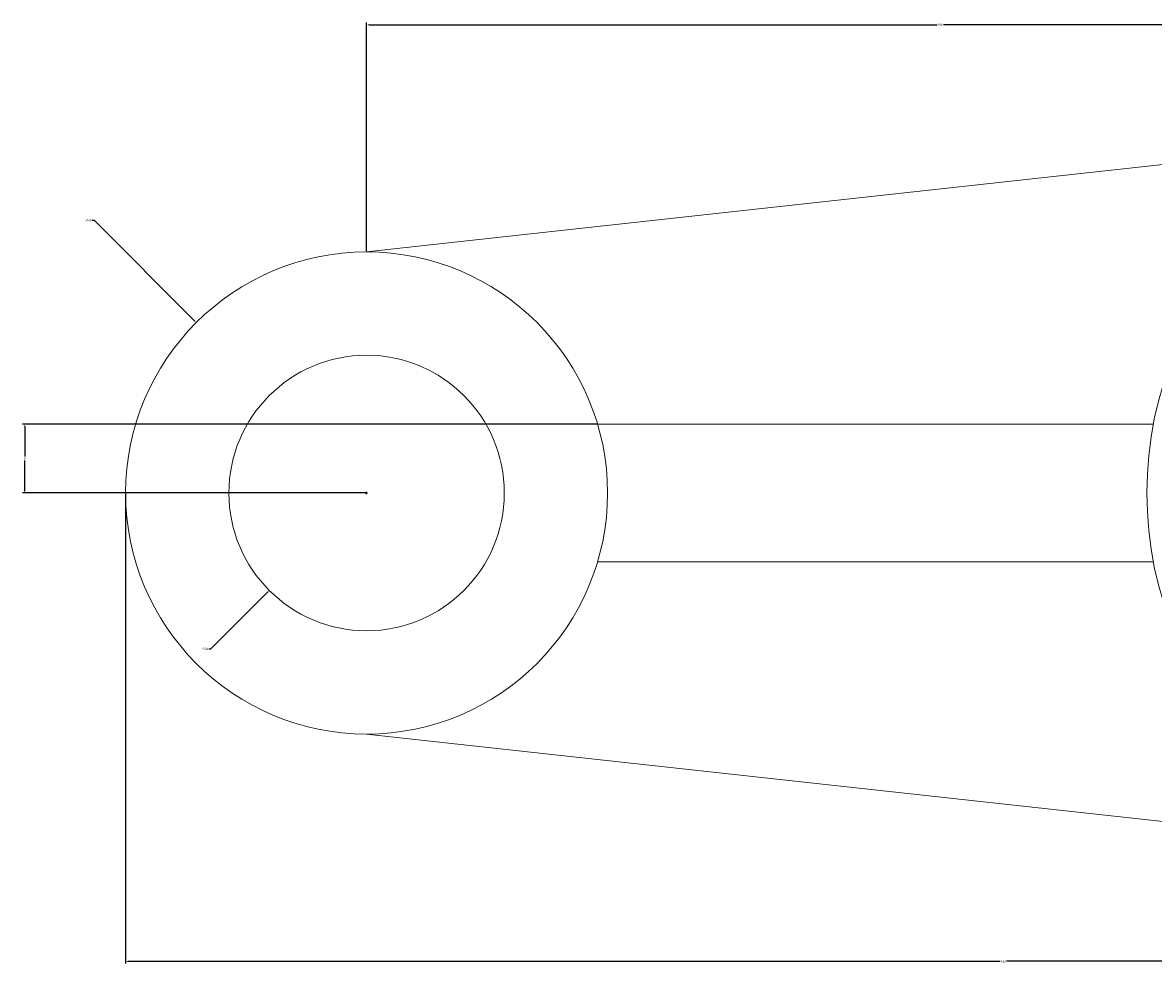
# Model space of a CAD drawing. Units: inches. Extents: x -47 to 120, y -20 to 62.
# Tile 1 of 2: x -47 to 52, y -20 to 62. Entities that reach past the tile are written whole.
import ezdxf

# ---------------------------------------------------------------- set-up
doc = ezdxf.new("R2010")
doc.units = ezdxf.units.IN
doc.header["$MEASUREMENT"] = 0
doc.layers.add('M-CONS', color=8, linetype='Continuous', lineweight=13)
doc.layers.add('M-DIMS', color=2, linetype='Continuous', lineweight=18)
doc.styles.get("Standard").update_dxf_attribs({"font": 'arial.ttf'})
doc.dimstyles.get("Standard").update_dxf_attribs({"dimtxt": 0.18, "dimasz": 0.18, "dimexe": 0.18, "dimexo": 0.0625, "dimgap": 0.09, "dimtad": 0, "dimtih": 1, "dimtoh": 1, "dimdec": 4, "dimzin": 0, "dimdsep": 46, "dimtxsty": 'Standard', "dimcen": 0.09, "dimadec": 0, "dimazin": 0, "dimtfac": 1, "dimtdec": 4, "dimtofl": 0, "dimtmove": 0, "dimatfit": 3, "dimfxl": 1, "dimtolj": 1, "dimtzin": 0, "dimarcsym": 0})

# ---------------------------------------------------------------- blocks, each defined once
blk = doc.blocks.new('*D1')
at = {"layer": 'Defpoints', "color": 0, "transparency": 16777216}
for p in [(-37.874, 20.605), (115.126, 20.605), (115.126, -20.195)]:
    blk.add_point(p, dxfattribs=at)
at = {"layer": 'M-DIMS', "color": 0, "lineweight": -2, "transparency": 16777216}
for p, q in [((-37.874, 20.542), (-37.874, -20.375)), ((115.126, 20.542), (115.126, -20.375)), ((-37.694, -20.195), (38.345, -20.195)), ((114.946, -20.195), (38.906, -20.195))]:
    blk.add_line(p, q, dxfattribs=at)
at = {"layer": 'M-DIMS', "color": 0, "transparency": 16777216}
for points in [[(-37.694, -20.165), (-37.694, -20.225), (-37.874, -20.195)], [(114.946, -20.165), (114.946, -20.225), (115.126, -20.195)]]:
    blk.add_solid(points, dxfattribs=at)
at = {"layer": 'M-DIMS', "color": 0, "transparency": 16777216, "insert": (38.626, -20.195), "char_height": 0.18, "attachment_point": 5}
blk.add_mtext('\\A1;153', dxfattribs=at)
blk = doc.blocks.new('*D2')
at = {"layer": 'Defpoints', "color": 0, "transparency": 16777216}
for p in [(83.126, 61.405), (83.126, 52.605), (-16.874, 41.605)]:
    blk.add_point(p, dxfattribs=at)
at = {"layer": 'M-DIMS', "color": 0, "lineweight": -2, "transparency": 16777216}
for p, q in [((-16.874, 41.667), (-16.874, 61.585)), ((-16.694, 61.405), (32.846, 61.405)), ((82.946, 61.405), (33.406, 61.405)), ((83.126, 52.667), (83.126, 61.585))]:
    blk.add_line(p, q, dxfattribs=at)
at = {"layer": 'M-DIMS', "color": 0, "transparency": 16777216}
for points in [[(-16.694, 61.435), (-16.694, 61.375), (-16.874, 61.405)], [(82.946, 61.435), (82.946, 61.375), (83.126, 61.405)]]:
    blk.add_solid(points, dxfattribs=at)
at = {"layer": 'M-DIMS', "color": 0, "transparency": 16777216, "insert": (33.126, 61.405), "char_height": 0.18, "attachment_point": 5}
blk.add_mtext('\\A1;100', dxfattribs=at)
blk = doc.blocks.new('*D6')
at = {"layer": 'Defpoints', "color": 0, "transparency": 16777216}
for p in [(-46.674, 26.605), (3.25, 26.605), (-16.874, 20.605)]:
    blk.add_point(p, dxfattribs=at)
at = {"layer": 'M-DIMS', "color": 0, "lineweight": -2, "transparency": 16777216}
for p, q in [((3.188, 26.605), (-46.854, 26.605)), ((-46.674, 26.425), (-46.674, 23.787)), ((-46.674, 20.785), (-46.674, 23.423)), ((-16.937, 20.605), (-46.854, 20.605))]:
    blk.add_line(p, q, dxfattribs=at)
at = {"layer": 'M-DIMS', "color": 0, "transparency": 16777216}
for points in [[(-46.704, 26.425), (-46.644, 26.425), (-46.674, 26.605)], [(-46.704, 20.785), (-46.644, 20.785), (-46.674, 20.605)]]:
    blk.add_solid(points, dxfattribs=at)
at = {"layer": 'M-DIMS', "color": 0, "transparency": 16777216, "insert": (-46.674, 23.605), "char_height": 0.18, "attachment_point": 5}
blk.add_mtext('\\A1;6', dxfattribs=at)
blk = doc.blocks.new('*D8')
at = {"layer": 'Defpoints', "color": 0, "transparency": 16777216}
for p in [(-31.724, 35.454), (-2.025, 5.756)]:
    blk.add_point(p, dxfattribs=at)
at = {"layer": 'M-DIMS', "color": 0, "lineweight": -2, "transparency": 16777216}
for p, q in [((-40.813, 44.363), (-40.633, 44.363)), ((-40.633, 44.363), (-31.851, 35.581)), ((-16.964, 20.605), (-16.784, 20.605)), ((-16.874, 20.515), (-16.874, 20.695))]:
    blk.add_line(p, q, dxfattribs=at)
at = {"layer": 'M-DIMS', "color": 0, "transparency": 16777216}
blk.add_solid([(-31.83, 35.602), (-31.872, 35.56), (-31.724, 35.454)], dxfattribs=at)
at = {"layer": 'M-DIMS', "color": 0, "transparency": 16777216, "insert": (-41.129, 44.363), "char_height": 0.18, "attachment_point": 5}
blk.add_mtext('\\A1;∅42', dxfattribs=at)
blk = doc.blocks.new('*D9')
at = {"layer": 'Defpoints', "color": 0, "transparency": 16777216}
for p in [(-8.388, 29.09), (-25.36, 12.12)]:
    blk.add_point(p, dxfattribs=at)
at = {"layer": 'M-DIMS', "color": 0, "lineweight": -2, "transparency": 16777216}
for p, q in [((-16.964, 20.605), (-16.784, 20.605)), ((-16.874, 20.515), (-16.874, 20.695)), ((-30.452, 7.029), (-25.487, 11.993)), ((-30.632, 7.029), (-30.452, 7.029))]:
    blk.add_line(p, q, dxfattribs=at)
at = {"layer": 'M-DIMS', "color": 0, "transparency": 16777216}
blk.add_solid([(-25.509, 12.014), (-25.466, 11.971), (-25.36, 12.12)], dxfattribs=at)
at = {"layer": 'M-DIMS', "color": 0, "transparency": 16777216, "insert": (-30.948, 7.029), "char_height": 0.18, "attachment_point": 5}
blk.add_mtext('\\A1;∅24', dxfattribs=at)

msp = doc.modelspace()

# ---------------------------------------------------------------- linework, layer by layer
at = {"layer": 'M-CONS'}
for p, q in [((-16.8743, 41.6047), (83.1257, 52.6047)), ((3.2504, 26.6047), (51.6933, 26.6047)), ((4.1257, 26.6047), (51.1257, 26.6047)), ((3.2504, 14.6047), (51.6933, 14.6047)), ((51.6933, 14.6047, 36), (3.2504, 14.6047, 23.8841)), ((4.1257, 14.6047), (51.1257, 14.6047)), ((-16.8743, -0.3953), (83.1257, -11.3953))]:
    msp.add_line(p, q, dxfattribs=at)
for centre, radius in [((83.1257, 20.6047), 32), ((-16.8743, 20.6047), 21), ((-16.8743, 20.6047), 12)]:
    msp.add_circle(centre, radius, dxfattribs=at)

# ---------------------------------------------------------------- dimensions: what is measured, and where the dimension line sits
at = {"layer": 'M-DIMS'}
for base, p1, p2, picture, middle in [((83.1257, 61.4047), (-16.8743, 41.6047), (83.1257, 52.6047), '*D2', (33.1257, 61.4047)), ((115.1257, -20.1953), (-37.8743, 20.6047), (115.1257, 20.6047), '*D1', (38.6257, -20.1953))]:
    dim = msp.add_linear_dim(base=base, p1=p1, p2=p2, dimstyle='Standard', override={"dimdec": 0, "dimlfac": 1, "dimrnd": 0, "dimzin": 0, "dimdsep": 46, "dimlunit": 2}, dxfattribs=at)
    dim.commit()
    dim.dimension.update_dxf_attribs({"geometry": picture, "text_midpoint": middle})
for p1, p2, picture, middle in [((-2.0248, 5.7557), (-31.7237, 35.4537), '*D8', (-41.1293, 44.3631)), ((-8.3885, 29.0895), (-25.36, 12.12), '*D9', (-30.948, 7.0291))]:
    dim = msp.add_diameter_dim_2p(p1=p1, p2=p2, dimstyle='Standard', override={"dimdec": 0, "dimlfac": 1, "dimrnd": 0, "dimzin": 0, "dimdsep": 46, "dimlunit": 2}, dxfattribs=at)
    dim.commit()
    dim.dimension.update_dxf_attribs({"geometry": picture, "text_midpoint": middle, "dimtype": 163})
dim = msp.add_linear_dim(base=(-46.6743, 26.6047), p1=(-16.8743, 20.6047), p2=(3.2504, 26.6047), angle=90, dimstyle='Standard', override={"dimdec": 0, "dimlfac": 1, "dimrnd": 0, "dimzin": 0, "dimdsep": 46, "dimlunit": 2}, dxfattribs=at)
dim.commit()
dim.dimension.update_dxf_attribs({"geometry": '*D6', "text_midpoint": (-46.6743, 23.6047)})

doc.saveas('drawing.dxf')
